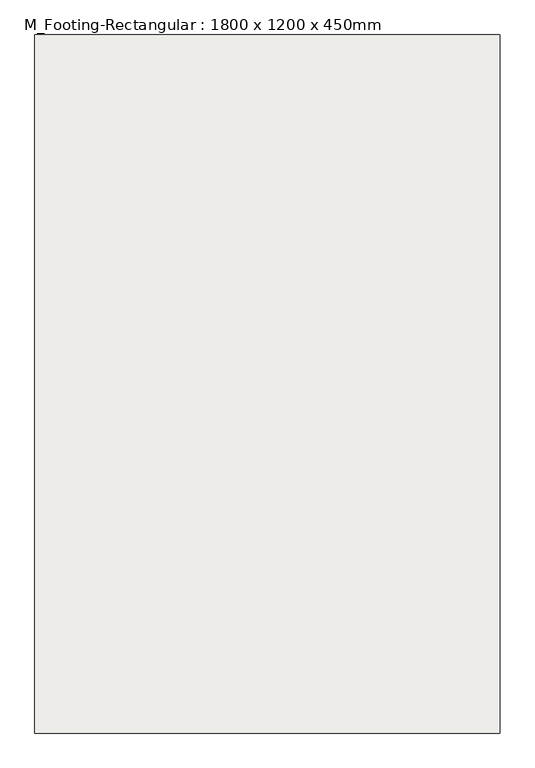
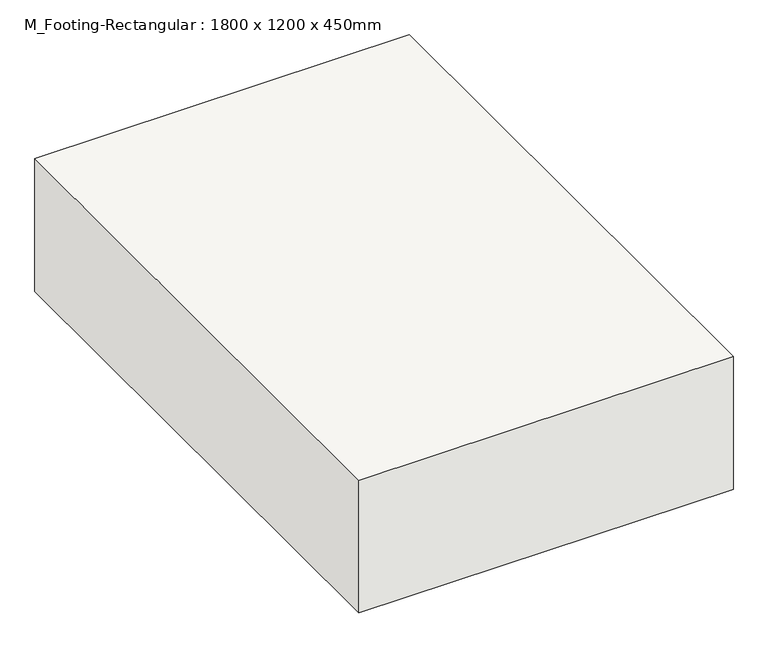
"""IFC4 building model written with IfcOpenShell, lengths in millimetres: slab geometry, M_Footing-Rectangular : 1800 x 1200 x 450mm."""

from ifc_helpers import new_model, si_unit, frame, origin, place, context, project, spatial, polyline, outline, extrude, source, transform, mapped, element, save


def m_footing_rectangular_1800_x_1200_x_450mm_16ba7ea5(model_context):
    return source(origin(), model_context, "Body", "SweptSolid", [
        extrude(outline(polyline([(600.0, 900.0), (600.0, -900.0), (-600.0, -900.0), (-600.0, 900.0), (600.0, 900.0)])), frame((0.0, 0.0, -450.0), z_axis=(0.0, 0.0, 1.0), x_axis=(1.0, 0.0, 0.0)), (0.0, 0.0, 1.0), 450.0),
    ])


if __name__ == "__main__":
    model = new_model("IFC4")
    model_context = context("Model", 3, world=origin())
    ifc_project = project(units=[si_unit("LENGTHUNIT", "METRE", prefix="MILLI")], contexts=[model_context])
    site = spatial("IfcSite", under=ifc_project)
    building = spatial("IfcBuilding", under=site)
    placement = place(None, origin())
    m_footing_rectangular_1800_x_1200_x_450mm_shape = m_footing_rectangular_1800_x_1200_x_450mm_16ba7ea5(model_context)
    element("IfcSlab", 1, ObjectType="M_Footing-Rectangular : 1800 x 1200 x 450mm", at=placement, inside=building, context=model_context, shape_type="MappedRepresentation", body=[
        mapped(m_footing_rectangular_1800_x_1200_x_450mm_shape, transform((0.0, 0.0, 0.0), x_axis=(1.0, 0.0, 0.0), y_axis=(0.0, 1.0, 0.0), z_axis=(0.0, 0.0, 1.0))),
    ])
    save(model, "model.ifc")

# Revit data of these elements
# Type "M_Footing-Rectangular : 1800 x 1200 x 450mm"
#   Width = 3' - 11.24409"
#   Length = 5' - 10.86614"
#   Foundation Thickness = 1' - 5.71654"
#   Structural Material [instance default] = Concrete, Cast-in-Place gray
#   Assembly Code = ""
# Element 1 (IfcSlab, "M_Footing-Rectangular : 1800 x 1200 x 450mm")
#   Materials on its faces: "Concrete, Cast-in-Place gray"
# Materials
#   "Concrete, Cast-in-Place gray": class "Concrete", colour RGB 192 192 192, transparency 0, Description = "Cast-in-place concrete", Cost = 0
